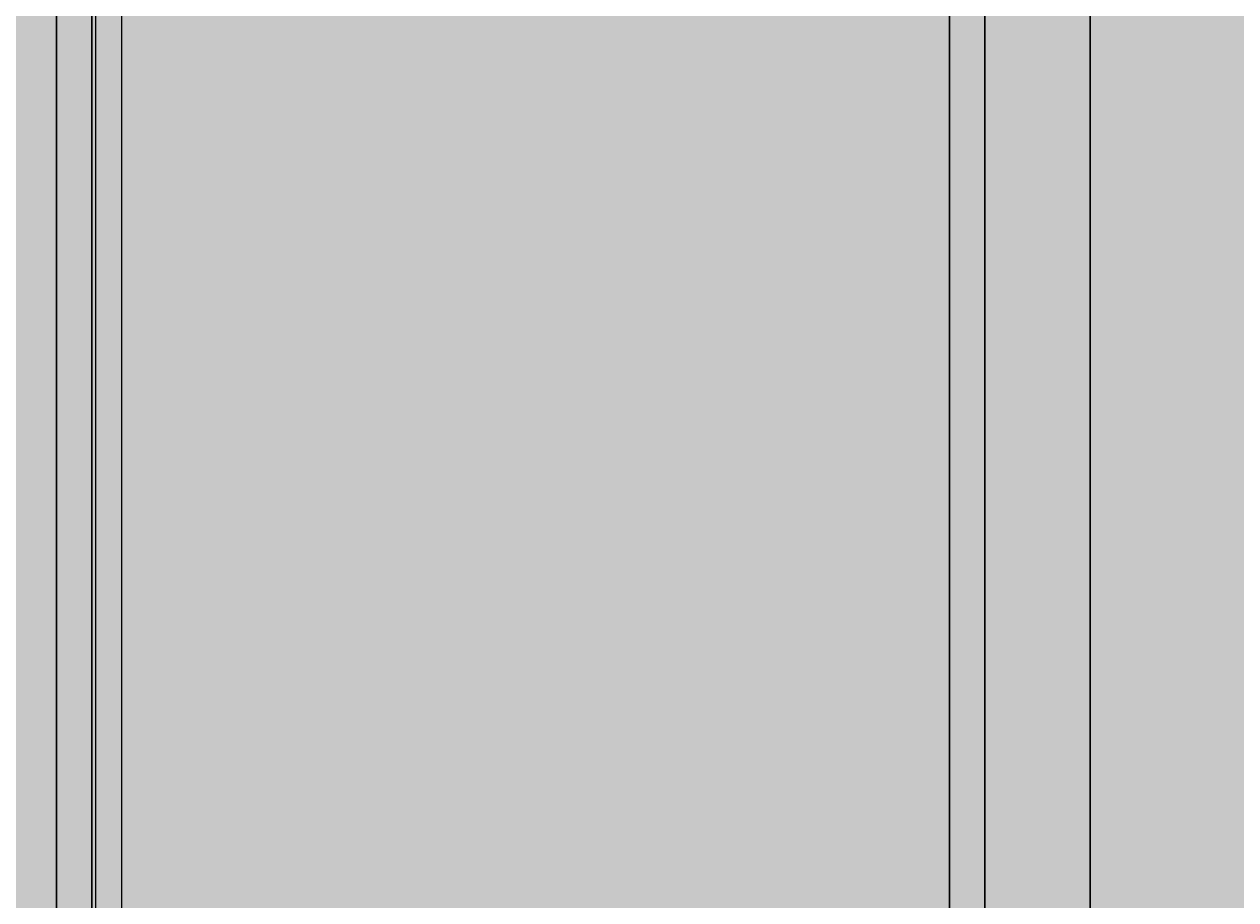
# Model space of a CAD drawing. Units: feet. Extents: x 2695 to 2912, y 795 to 1139.
# Tile 19 of 83: x 2808 to 2843, y 820 to 845. Entities that reach past the tile are written whole.
import ezdxf

# ---------------------------------------------------------------- set-up
doc = ezdxf.new("R2010")
doc.units = ezdxf.units.FT
for name, color, linetype, lineweight in [('A-ANNO-DIMS', 2, 'Continuous', 18), ('A-DOOR', 3, 'Continuous', 25), ('A-DOOR-PATT', 33, 'Continuous', 13), ('A-ELEV-PATT', 252, 'Continuous', 13)]:
    doc.layers.add(name, color=color, linetype=linetype, lineweight=lineweight)
doc.styles.get("Standard").update_dxf_attribs({"font": 'arial.ttf'})
doc.dimstyles.get("Standard").update_dxf_attribs({"dimtxt": 0.18, "dimasz": 0.18, "dimexe": 0.18, "dimexo": 0.0625, "dimgap": 0.09, "dimtad": 0, "dimtih": 1, "dimtoh": 1, "dimdec": 1, "dimzin": 0, "dimdsep": 46, "dimlunit": 3, "dimtxsty": 'Standard', "dimcen": 0.09, "dimadec": 0, "dimazin": 0, "dimtfac": 1, "dimtdec": 1, "dimtofl": 0, "dimtmove": 0, "dimatfit": 3, "dimfxl": 1, "dimtolj": 1, "dimtzin": 0, "dimarcsym": 0})

# ---------------------------------------------------------------- blocks, each defined once
blk = doc.blocks.new('*D13')
at = {"layer": 'A-ANNO-DIMS', "color": 0, "lineweight": -2, "transparency": 16777216}
for p, q in [((2758.214, 874.857), (2911.424, 874.857)), ((2911.244, 874.677), (2911.244, 843.076)), ((2911.244, 811.111), (2911.244, 842.712)), ((2890.699, 810.931), (2911.424, 810.931))]:
    blk.add_line(p, q, dxfattribs=at)
at = {"layer": 'A-ANNO-DIMS', "color": 0, "transparency": 16777216}
for points in [[(2911.214, 874.677), (2911.274, 874.677), (2911.244, 874.857)], [(2911.214, 811.111), (2911.274, 811.111), (2911.244, 810.931)]]:
    blk.add_solid(points, dxfattribs=at)
at = {"layer": 'Defpoints', "color": 0, "transparency": 16777216}
for p in [(2758.151, 874.857), (2911.244, 874.857), (2890.636, 810.931)]:
    blk.add_point(p, dxfattribs=at)
at = {"layer": 'A-ANNO-DIMS', "color": 0, "transparency": 16777216, "insert": (2911.244, 842.894), "char_height": 0.18, "attachment_point": 5}
blk.add_mtext('\\A1;63.93', dxfattribs=at)
blk = doc.blocks.new('*D52')
at = {"layer": 'A-ANNO-DIMS', "color": 0, "lineweight": -2, "transparency": 16777216}
for p, q in [((2810.041, 936.868), (2810.041, 794.976)), ((2810.789, 936.868), (2810.789, 794.976)), ((2809.861, 795.156), (2809.681, 795.156)), ((2810.969, 795.156), (2811.149, 795.156))]:
    blk.add_line(p, q, dxfattribs=at)
at = {"layer": 'A-ANNO-DIMS', "color": 0, "transparency": 16777216}
for points in [[(2809.861, 795.186), (2809.861, 795.126), (2810.041, 795.156)], [(2810.969, 795.186), (2810.969, 795.126), (2810.789, 795.156)]]:
    blk.add_solid(points, dxfattribs=at)
at = {"layer": 'Defpoints', "color": 0, "transparency": 16777216}
for p in [(2810.041, 936.931), (2810.789, 936.931), (2810.789, 795.156)]:
    blk.add_point(p, dxfattribs=at)
at = {"layer": 'A-ANNO-DIMS', "color": 0, "transparency": 16777216, "insert": (2810.415, 795.156), "char_height": 0.18, "attachment_point": 5}
blk.add_mtext('\\A1;0.75', dxfattribs=at)

msp = doc.modelspace()

# ---------------------------------------------------------------- hatches: boundary and pattern name
at = {"layer": 'A-DOOR-PATT'}
h = msp.add_hatch(color=256, dxfattribs=at)
h.set_gradient(color1=(211, 185, 150), color2=(211, 185, 150))
h.paths.add_polyline_path([(2805.9398, 905.5143), (2773.5029, 905.5143), (2773.5029, 810.9306), (2776.4999, 810.9306), (2776.4999, 902.5174), (2802.9429, 902.5174), (2802.9429, 810.9306), (2805.9398, 810.9306)])
h.paths.add_polyline_path([(2803.9681, 874.1057), (2805.0538, 874.1057), (2805.0538, 846.2857), (2803.9681, 846.2857)], flags=16)
h.paths.add_polyline_path([(2838.3767, 905.5143), (2805.9398, 905.5143), (2805.9398, 810.9306), (2808.9368, 810.9306), (2808.9368, 902.5174), (2835.3798, 902.5174), (2835.3798, 810.9306), (2838.3767, 810.9306)])
h = msp.add_hatch(color=256, dxfattribs=at)
h.set_gradient(color1=(211, 185, 150), color2=(211, 185, 150))
h.paths.add_polyline_path([(2777.5029, 901.5143), (2801.9398, 901.5143), (2801.9398, 810.9306), (2802.9429, 810.9306), (2802.9429, 902.5174), (2776.4999, 902.5174), (2776.4999, 810.9306), (2777.5029, 810.9306)])
h.paths.add_polyline_path([(2809.9398, 901.5143), (2834.3767, 901.5143), (2834.3767, 810.9306), (2835.3798, 810.9306), (2835.3798, 902.5174), (2808.9368, 902.5174), (2808.9368, 810.9306), (2809.9398, 810.9306)])
h = msp.add_hatch(color=256, dxfattribs=at)
h.set_gradient(color1=(173, 221, 247), color2=(173, 221, 247))
h.paths.add_polyline_path([(2801.9398, 901.5143), (2777.5029, 901.5143), (2777.5029, 810.9306), (2801.9398, 810.9306)])
h.paths.add_polyline_path([(2834.3767, 901.5143), (2809.9398, 901.5143), (2809.9398, 810.9306), (2834.3767, 810.9306)])
at = {"layer": 'A-ELEV-PATT'}
h = msp.add_hatch(color=256, dxfattribs=at)
h.set_gradient(color1=(147, 149, 152), color2=(147, 149, 152), tint=1)
h.paths.add_polyline_path([(2770.6361, 1118.4096), (2710.6361, 1118.4096), (2710.6361, 1062.9306), (2770.6361, 1062.9306)])
h.paths.add_polyline_path([(2890.6361, 1103.3378), (2770.6361, 1103.3378), (2770.6361, 1062.9306), (2890.6361, 1062.9306)])
h.paths.add_polyline_path([(2730.7081, 1048.1052), (2755.1125, 1048.1052), (2755.1125, 936.9306), (2770.6361, 936.9306), (2770.6361, 1050.3105), (2715.8852, 1050.3105), (2715.8852, 936.9306), (2730.7081, 936.9306)])
h.paths.add_polyline_path([(2890.6361, 1050.3105), (2770.6361, 1050.3105), (2770.6361, 971.9673), (2778.0341, 971.9673), (2778.0341, 1020.8235), (2843.575, 1020.8235), (2843.575, 971.9673), (2890.6361, 971.9673)])
h.paths.add_polyline_path([(2888.1882, 970.7156), (2843.575, 970.7156), (2843.575, 964.8267), (2888.1882, 964.8267)])
h.paths.add_polyline_path([(2888.1882, 964.1328), (2843.575, 964.1328), (2843.575, 956.614), (2888.1882, 956.614)])
h.paths.add_polyline_path([(2888.1882, 955.9202), (2843.575, 955.9202), (2843.575, 949.2892), (2888.1882, 949.2892)])
h.paths.add_polyline_path([(2888.1882, 948.5954), (2843.575, 948.5954), (2843.575, 941.3507), (2888.1882, 941.3507)])
h.paths.add_polyline_path([(2888.1882, 940.6569), (2843.575, 940.6569), (2843.575, 936.9306), (2888.1882, 936.9306)])
h.paths.add_polyline_path([(2890.6361, 970.7156), (2888.9368, 970.7156), (2888.9368, 964.8267), (2890.6361, 964.8267)])
h.paths.add_polyline_path([(2890.6361, 964.1328), (2888.9368, 964.1328), (2888.9368, 956.614), (2890.6361, 956.614)])
h.paths.add_polyline_path([(2890.6361, 955.9202), (2888.9368, 955.9202), (2888.9368, 949.2892), (2890.6361, 949.2892)])
h.paths.add_polyline_path([(2890.6361, 940.6569), (2888.9368, 940.6569), (2888.9368, 936.9306), (2890.6361, 936.9306)])
h.paths.add_polyline_path([(2890.6361, 948.5954), (2888.9368, 948.5954), (2888.9368, 941.3507), (2890.6361, 941.3507)])
h.paths.add_polyline_path([(2772.5216, 970.7156), (2770.6361, 970.7156), (2770.6361, 964.8267), (2772.5216, 964.8267)])
h.paths.add_polyline_path([(2772.5216, 964.1328), (2770.6361, 964.1328), (2770.6361, 956.614), (2772.5216, 956.614)])
h.paths.add_polyline_path([(2772.5216, 955.9202), (2770.6361, 955.9202), (2770.6361, 949.2892), (2772.5216, 949.2892)])
h.paths.add_polyline_path([(2772.5216, 948.5954), (2770.6361, 948.5954), (2770.6361, 941.3507), (2772.5216, 941.3507)])
h.paths.add_polyline_path([(2772.5216, 940.6569), (2770.6361, 940.6569), (2770.6361, 936.9306), (2772.5216, 936.9306)])
h.paths.add_polyline_path([(2778.0341, 940.6569), (2773.2702, 940.6569), (2773.2702, 936.9306), (2778.0341, 936.9306)])
h.paths.add_polyline_path([(2778.0341, 970.7156), (2773.2702, 970.7156), (2773.2702, 964.8267), (2778.0341, 964.8267)])
h.paths.add_polyline_path([(2778.0341, 964.1328), (2773.2702, 964.1328), (2773.2702, 956.614), (2778.0341, 956.614)])
h.paths.add_polyline_path([(2778.0341, 955.9202), (2773.2702, 955.9202), (2773.2702, 949.2892), (2778.0341, 949.2892)])
h.paths.add_polyline_path([(2778.0341, 948.5954), (2773.2702, 948.5954), (2773.2702, 941.3507), (2778.0341, 941.3507)])
h.paths.add_polyline_path([(2810.0407, 940.6569), (2780.0341, 940.6569), (2780.0341, 936.9306), (2810.0407, 936.9306)])
h.paths.add_polyline_path([(2890.6361, 924.3105), (2770.6361, 924.3105), (2770.6361, 810.9306), (2773.5029, 810.9306), (2773.5029, 905.5143), (2805.9398, 905.5143), (2838.3767, 905.5143), (2838.3767, 810.9306), (2890.6361, 810.9306)])

# ---------------------------------------------------------------- linework, layer by layer
at = {"layer": 'A-DOOR'}
for points in [[(2773.5029, 905.5143), (2838.3767, 905.5143), (2838.3767, 810.9306), (2773.5029, 810.9306)], [(2808.9368, 902.5174), (2835.3798, 902.5174), (2835.3798, 810.9306), (2808.9368, 810.9306)], [(2809.9398, 901.5143), (2834.3767, 901.5143), (2834.3767, 810.9306), (2809.9398, 810.9306)]]:
    msp.add_lwpolyline(points, close=True, dxfattribs=at)
for points in [[(2838.3767, 810.9306), (2838.3767, 905.5143), (2805.9398, 905.5143), (2805.9398, 810.9306)], [(2835.3798, 810.9306), (2835.3798, 902.5174), (2808.9368, 902.5174), (2808.9368, 810.9306)], [(2834.3767, 810.9306), (2834.3767, 901.5143), (2809.9398, 901.5143), (2809.9398, 810.9306)]]:
    msp.add_lwpolyline(points, dxfattribs=at)

# ---------------------------------------------------------------- dimensions: what is measured, and where the dimension line sits
at = {"layer": 'A-ANNO-DIMS'}
dim = msp.add_linear_dim(base=(2810.7893, 795.1556), p1=(2810.0407, 936.9306), p2=(2810.7893, 936.9306), dimstyle='Standard', override={"dimdec": 2, "dimlfac": 1, "dimrnd": 0, "dimzin": 0, "dimdsep": 46, "dimlunit": 2}, dxfattribs=at)
dim.commit()
dim.dimension.update_dxf_attribs({"geometry": '*D52', "text_midpoint": (2810.415, 795.1556)})
dim = msp.add_linear_dim(base=(2911.2444, 874.8571), p1=(2890.6361, 810.9306), p2=(2758.1515, 874.8571), angle=90, dimstyle='Standard', override={"dimdec": 2, "dimlfac": 1, "dimrnd": 0, "dimzin": 0, "dimdsep": 46, "dimlunit": 2}, dxfattribs=at)
dim.commit()
dim.dimension.update_dxf_attribs({"geometry": '*D13', "text_midpoint": (2911.2444, 842.8938)})

doc.saveas('drawing.dxf')
